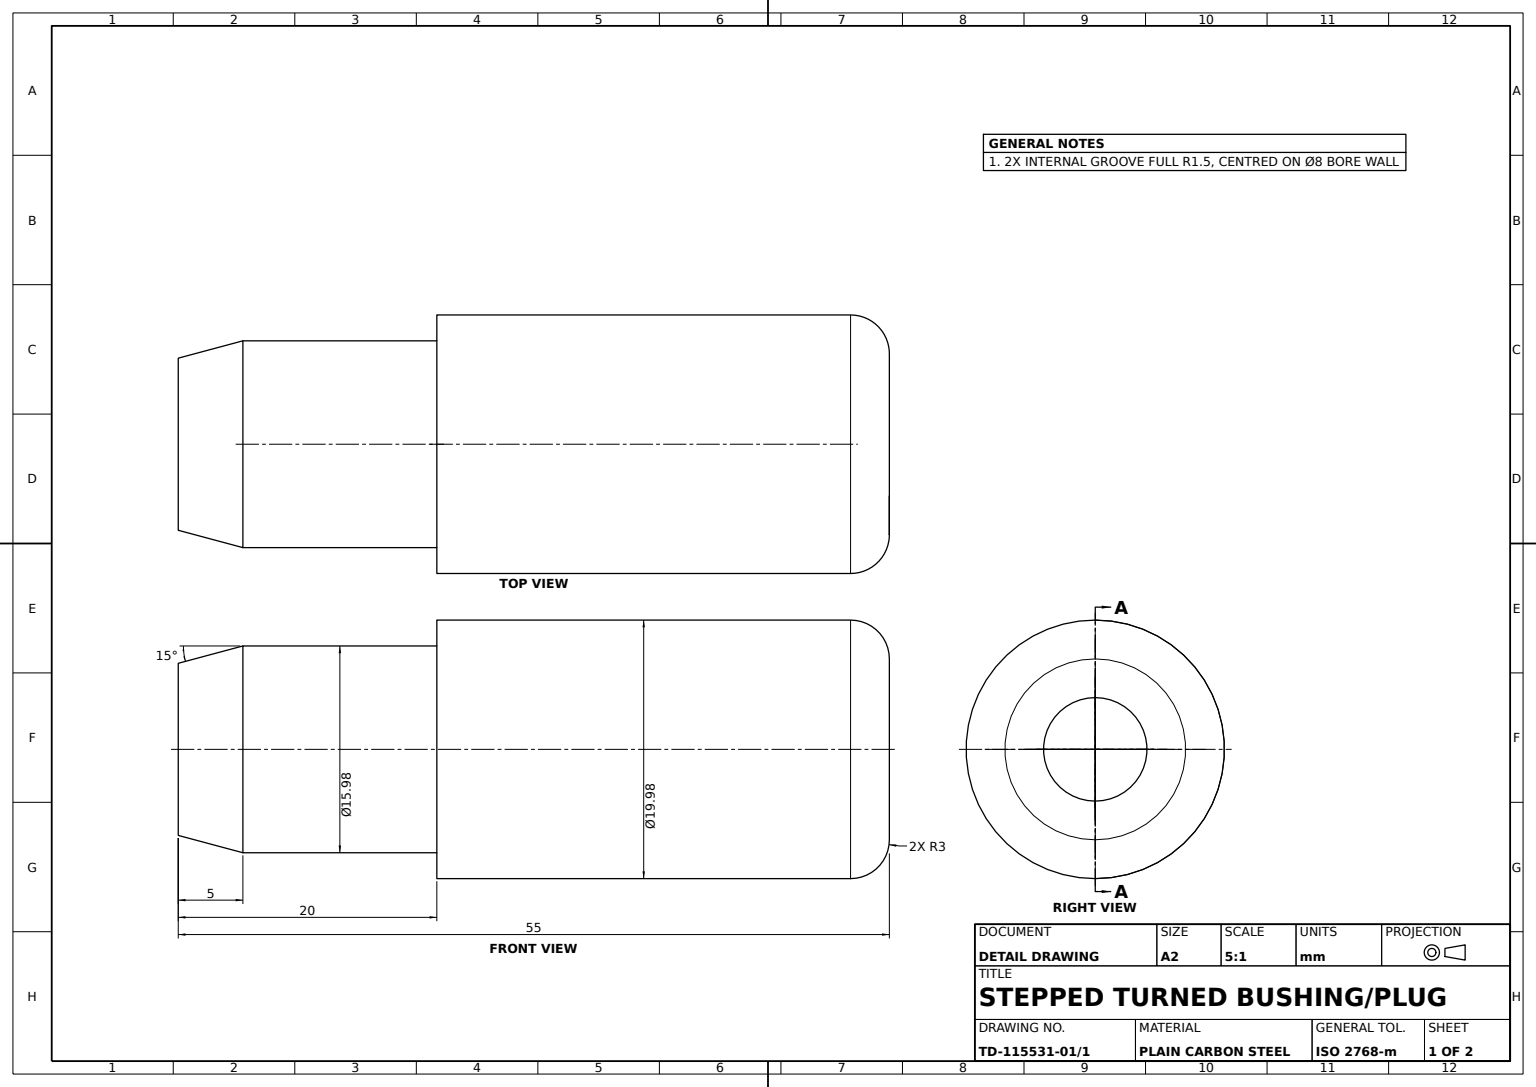
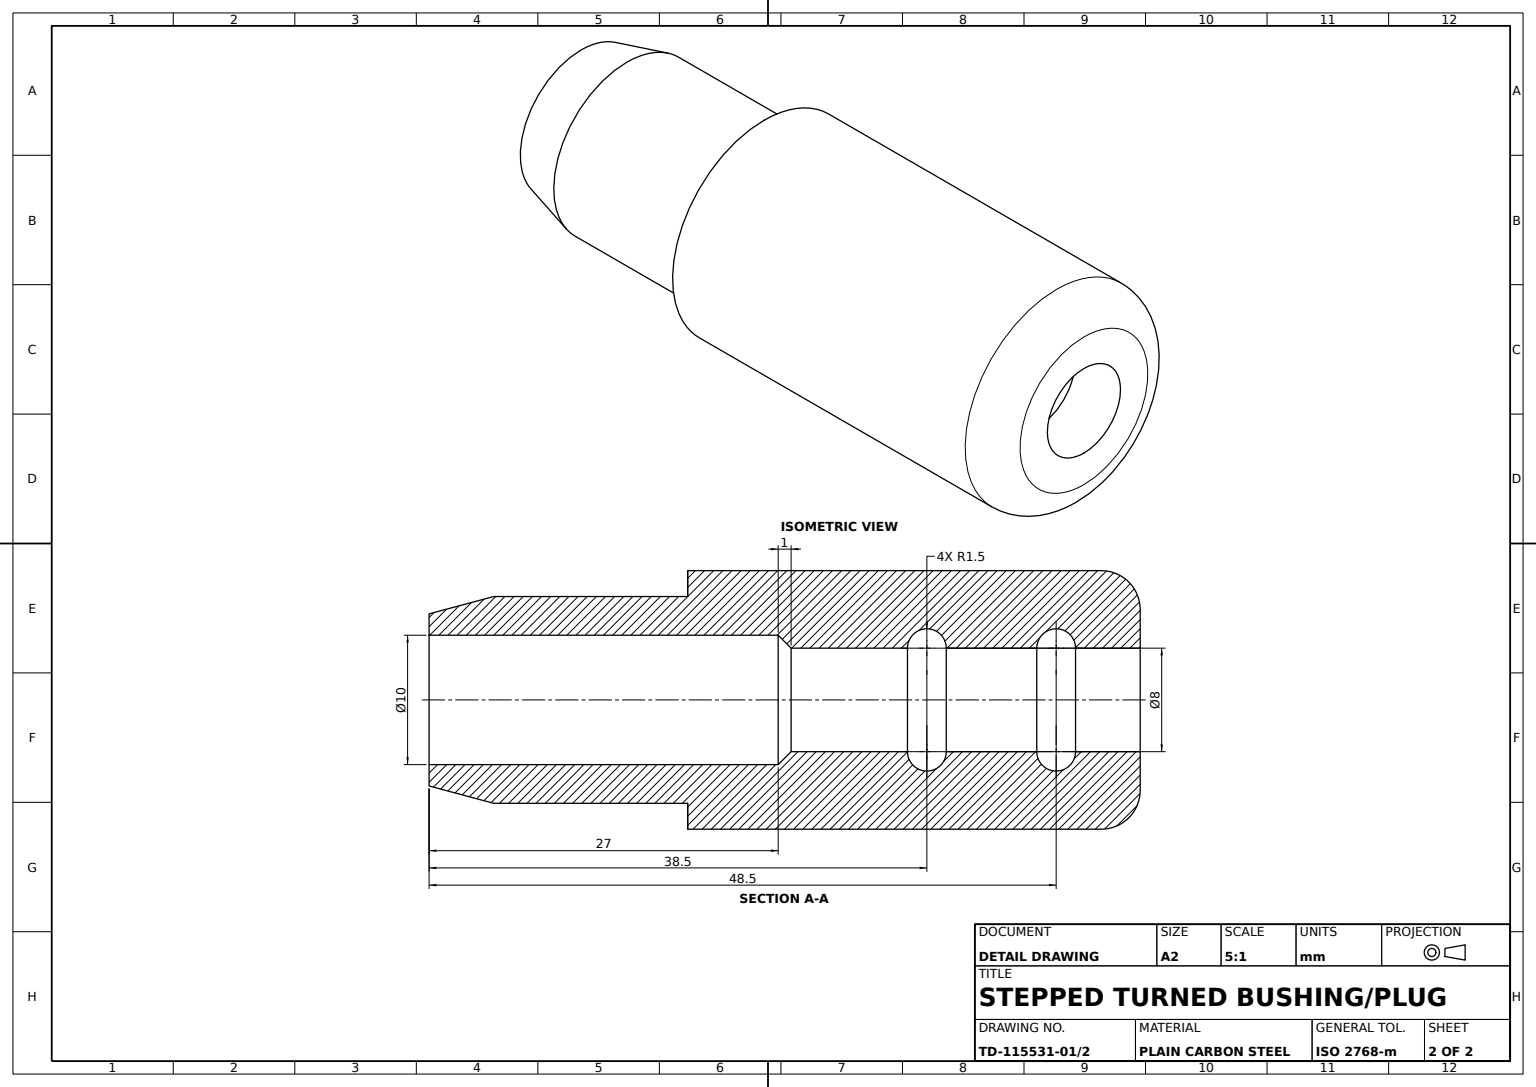
from build123d import *


with BuildPart() as part:
    # Pin Profile Sketch → Pin Body Revolve (revolve)
    with BuildSketch(Plane.XY, mode=Mode.PRIVATE) as pin_body_revolve_sk:
        with BuildLine():
            Line((5, 0), (5, 27))
            Line((5, 27), (4, 28))
            Line((4, 28), (4, 37))
            ThreePointArc((4, 37), (5.5, 38.5), (4, 40))
            Line((4, 40), (4, 47))
            ThreePointArc((4, 47), (5.5, 48.5), (4, 50))
            Line((4, 50), (4, 55))
            Line((4, 55), (6.989745962, 55))
            ThreePointArc((6.989745962, 55), (9.111066306, 54.121320344), (9.989745962, 52))
            Line((9.989745962, 52), (9.989745962, 20))
            Line((9.989745962, 20), (7.989745962, 20))
            Line((7.989745962, 20), (7.989745962, 5))
            Line((7.989745962, 5), (6.65, 0))
            Line((6.65, 0), (5, 0))
        make_face()
    revolve(pin_body_revolve_sk.sketch.rotate(Axis((0, 37.717557252, 0), (0, -1, 0)), 180), axis=Axis((0, 37.717557252, 0), (0, -1, 0)))


solid = part.part
